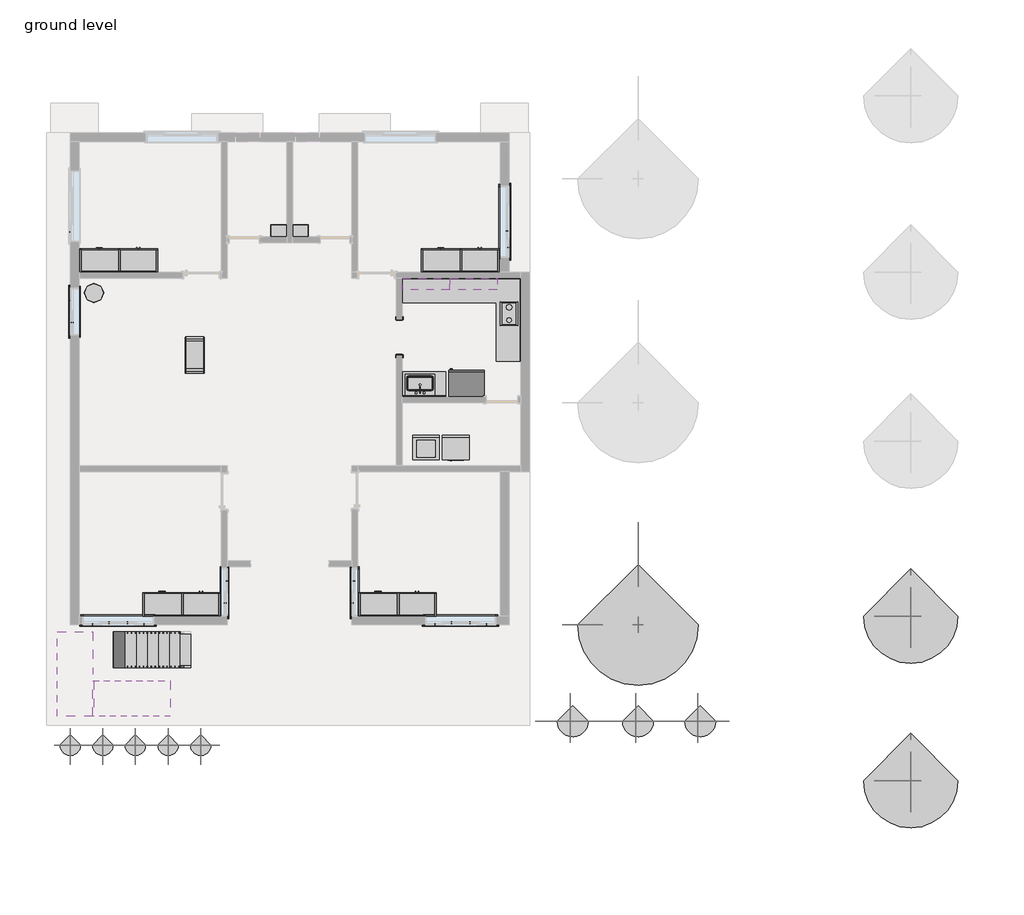
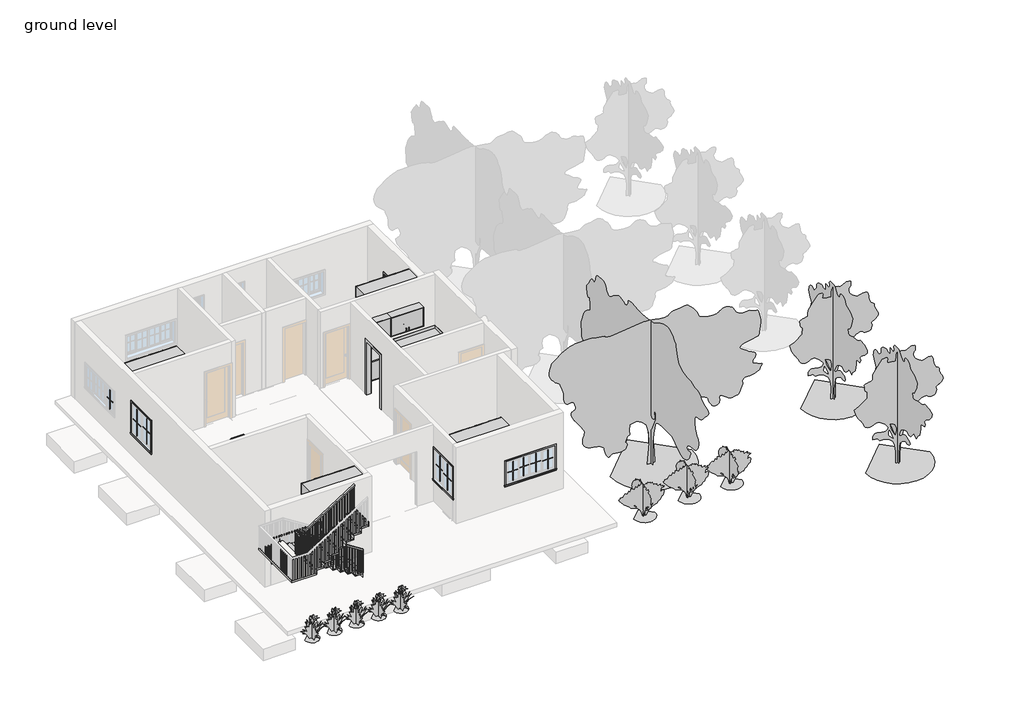
# One storey, part 3 of 4: 33 proxies, 15 furniture elements, 11 geographic elements, 3 flow terminals, 2 stair flights, 1 railing, 1 slab.
"""IFC4 building model written with IfcOpenShell, lengths in millimetres."""

from ifc_helpers import new_model, si_unit, frame, origin, place, context, project, spatial, polyline, outline, extrude, faceted_brep, transform, mapped, element, save
from components import proxy_3c1fa1d0, proxy_97c73763, muntin_pattern_2x2_muntin_pattern_2x2_c2d27229, muntin_pattern_2x2_muntin_pattern_2x2_cf37b409, muntin_pattern_2x2_muntin_pattern_2x2_31a16349, proxy_7dd6dadb, trim_window_exterior_flat_with_sill_ac84ebb5, trim_window_exterior_flat_with_sill_7cfdd449, trim_window_exterior_flat_with_sill_3c945769, trim_window_interior_flat_picture_frame_caf2db4f, trim_window_interior_flat_picture_frame_f1e0b15b, trim_window_interior_flat_picture_frame_0edfbaa2, proxy_e75280ca, flow_terminal_7145266d, flow_terminal_4d548711, furniture_2dca108f, furniture_65fa61b5, furniture_1wardrobe_6271_1wardrobe_6271_4dd35231, furniture_3428e43d, furniture_bf8a676d, furniture_97fe820d, furniture_a6d59748, furniture_f5a42f9b, furniture_9d41381f, furniture_ea954fa4, rpc_plant_tropical_55f6ff97, rpc_plant_tropical_6475341c, rpc_tree_deciduous_common_apple_20_2cf08d23, rpc_tree_deciduous_japanese_cherry_15_e499737d, non_monolithic_landing_d7d9d8c2, stair_flight_7bdf39d0, stair_flight_d241fc77

model = new_model("IFC4")

# Units and contexts
model_context = context("Model", 3, world=origin())
ifc_project = project(units=[si_unit("LENGTHUNIT", "METRE", prefix="MILLI")], contexts=[model_context])

# Site, building, storey
site = spatial("IfcSite", under=ifc_project)
building = spatial("IfcBuilding", under=site)
storey = spatial("IfcBuildingStorey", under=building, Name="ground level", Elevation=609.6)

# Proxies
placement = place(None, origin())
proxy_shape = proxy_3c1fa1d0(model_context)
element("IfcBuildingElementProxy", 1, Name="Cook Top-2 Unit : 12\" x 18\" 2", ObjectType="Cook Top-2 Unit : 12\" x 18\" 2", at=placement, inside=storey, context=model_context, shape_type="MappedRepresentation", body=[
    mapped(proxy_shape, transform((-1440.8124084, 5502.3713848, 609.6), x_axis=(1.0, 0.0, 0.0), y_axis=(0.0, 1.0, 0.0), z_axis=(0.0, 0.0, 1.0))),
])
proxy_2_shape = proxy_97c73763(model_context)
element("IfcBuildingElementProxy", 2, Name="Dryer : 27\" x 25\" x 35\"", ObjectType="Dryer : 27\" x 25\" x 35\"", at=placement, inside=storey, context=model_context, shape_type="MappedRepresentation", body=[
    mapped(proxy_2_shape, transform((-3115.1998647, 1776.2351766, 609.6), x_axis=(1.0, 0.0, 0.0), y_axis=(0.0, 1.0, 0.0), z_axis=(0.0, 0.0, 1.0))),
])
muntin_pattern_2x2_muntin_pattern_2x2_shape = muntin_pattern_2x2_muntin_pattern_2x2_c2d27229(model_context)
element("IfcBuildingElementProxy", 3, Name="Muntin Pattern_2x2 : Muntin Pattern_2x2", ObjectType="Muntin Pattern_2x2 : Muntin Pattern_2x2", at=placement, inside=storey, context=model_context, shape_type="MappedRepresentation", body=[
    mapped(muntin_pattern_2x2_muntin_pattern_2x2_shape, transform((-12588.2374084, 5299.2336804, 1606.55), x_axis=(0.0, -1.0, 0.0), y_axis=(1.0, 0.0, 0.0), z_axis=(0.0, 0.0, 1.0))),
])
element("IfcBuildingElementProxy", 4, Name="Muntin Pattern_2x2 : Muntin Pattern_2x2", ObjectType="Muntin Pattern_2x2 : Muntin Pattern_2x2", at=placement, inside=storey, context=model_context, shape_type="MappedRepresentation", body=[
    mapped(muntin_pattern_2x2_muntin_pattern_2x2_shape, transform((-12632.6874084, 5867.5586804, 1606.55), x_axis=(0.0, -1.0, 0.0), y_axis=(1.0, 0.0, 0.0), z_axis=(0.0, 0.0, 1.0))),
])
muntin_pattern_2x2_muntin_pattern_2x2_2_shape = muntin_pattern_2x2_muntin_pattern_2x2_cf37b409(model_context)
element("IfcBuildingElementProxy", 5, Name="Muntin Pattern_2x2 : Muntin Pattern_2x2", ObjectType="Muntin Pattern_2x2 : Muntin Pattern_2x2", at=placement, inside=storey, context=model_context, shape_type="MappedRepresentation", body=[
    mapped(muntin_pattern_2x2_muntin_pattern_2x2_2_shape, transform((-8657.5874084, -1908.0163196, 1606.55), x_axis=(0.0, -1.0, 0.0), y_axis=(1.0, 0.0, 0.0), z_axis=(0.0, 0.0, 1.0))),
])
element("IfcBuildingElementProxy", 6, Name="Muntin Pattern_2x2 : Muntin Pattern_2x2", ObjectType="Muntin Pattern_2x2 : Muntin Pattern_2x2", at=placement, inside=storey, context=model_context, shape_type="MappedRepresentation", body=[
    mapped(muntin_pattern_2x2_muntin_pattern_2x2_2_shape, transform((-8613.1374084, -1339.6913196, 1606.55), x_axis=(0.0, -1.0, 0.0), y_axis=(1.0, 0.0, 0.0), z_axis=(0.0, 0.0, 1.0))),
])
element("IfcBuildingElementProxy", 7, Name="Muntin Pattern_2x2 : Muntin Pattern_2x2", ObjectType="Muntin Pattern_2x2 : Muntin Pattern_2x2", at=placement, inside=storey, context=model_context, shape_type="MappedRepresentation", body=[
    mapped(muntin_pattern_2x2_muntin_pattern_2x2_2_shape, transform((-5349.2374084, -1339.6913196, 1606.55), x_axis=(0.0, 1.0, 0.0), y_axis=(-1.0, 0.0, 0.0), z_axis=(0.0, 0.0, 1.0))),
])
element("IfcBuildingElementProxy", 8, Name="Muntin Pattern_2x2 : Muntin Pattern_2x2", ObjectType="Muntin Pattern_2x2 : Muntin Pattern_2x2", at=placement, inside=storey, context=model_context, shape_type="MappedRepresentation", body=[
    mapped(muntin_pattern_2x2_muntin_pattern_2x2_2_shape, transform((-5393.6874084, -1908.0163196, 1606.55), x_axis=(0.0, 1.0, 0.0), y_axis=(-1.0, 0.0, 0.0), z_axis=(0.0, 0.0, 1.0))),
])
muntin_pattern_2x2_muntin_pattern_2x2_3_shape = muntin_pattern_2x2_muntin_pattern_2x2_31a16349(model_context)
element("IfcBuildingElementProxy", 9, Name="Muntin Pattern_2x2 : Muntin Pattern_2x2", ObjectType="Muntin Pattern_2x2 : Muntin Pattern_2x2", at=placement, inside=storey, context=model_context, shape_type="MappedRepresentation", body=[
    mapped(muntin_pattern_2x2_muntin_pattern_2x2_3_shape, transform((-12632.6874084, 7634.4461804, 1606.55), x_axis=(0.0, 1.0, 0.0), y_axis=(-1.0, 0.0, 0.0), z_axis=(0.0, 0.0, 1.0))),
])
element("IfcBuildingElementProxy", 10, Name="Muntin Pattern_2x2 : Muntin Pattern_2x2", ObjectType="Muntin Pattern_2x2 : Muntin Pattern_2x2", at=placement, inside=storey, context=model_context, shape_type="MappedRepresentation", body=[
    mapped(muntin_pattern_2x2_muntin_pattern_2x2_3_shape, transform((-1418.5874084, 7659.8461804, 1606.55), x_axis=(0.0, -1.0, 0.0), y_axis=(1.0, 0.0, 0.0), z_axis=(0.0, 0.0, 1.0))),
])
element("IfcBuildingElementProxy", 11, Name="Muntin Pattern_2x2 : Muntin Pattern_2x2", ObjectType="Muntin Pattern_2x2 : Muntin Pattern_2x2", at=placement, inside=storey, context=model_context, shape_type="MappedRepresentation", body=[
    mapped(muntin_pattern_2x2_muntin_pattern_2x2_3_shape, transform((-1374.1374084, 7234.3961804, 1606.55), x_axis=(0.0, -1.0, 0.0), y_axis=(1.0, 0.0, 0.0), z_axis=(0.0, 0.0, 1.0))),
])
element("IfcBuildingElementProxy", 12, Name="Muntin Pattern_2x2 : Muntin Pattern_2x2", ObjectType="Muntin Pattern_2x2 : Muntin Pattern_2x2", at=placement, inside=storey, context=model_context, shape_type="MappedRepresentation", body=[
    mapped(muntin_pattern_2x2_muntin_pattern_2x2_3_shape, transform((-1948.8124084, -2458.8788196, 1606.55), x_axis=(-1.0, 0.0, 0.0), y_axis=(0.0, -1.0, 0.0), z_axis=(0.0, 0.0, 1.0))),
])
element("IfcBuildingElementProxy", 13, Name="Muntin Pattern_2x2 : Muntin Pattern_2x2", ObjectType="Muntin Pattern_2x2 : Muntin Pattern_2x2", at=placement, inside=storey, context=model_context, shape_type="MappedRepresentation", body=[
    mapped(muntin_pattern_2x2_muntin_pattern_2x2_3_shape, transform((-2374.2624084, -2414.4288196, 1606.55), x_axis=(-1.0, 0.0, 0.0), y_axis=(0.0, -1.0, 0.0), z_axis=(0.0, 0.0, 1.0))),
])
element("IfcBuildingElementProxy", 14, Name="Muntin Pattern_2x2 : Muntin Pattern_2x2", ObjectType="Muntin Pattern_2x2 : Muntin Pattern_2x2", at=placement, inside=storey, context=model_context, shape_type="MappedRepresentation", body=[
    mapped(muntin_pattern_2x2_muntin_pattern_2x2_3_shape, transform((-2844.1624084, -2414.4288196, 1606.55), x_axis=(-1.0, 0.0, 0.0), y_axis=(0.0, -1.0, 0.0), z_axis=(0.0, 0.0, 1.0))),
])
element("IfcBuildingElementProxy", 15, Name="Muntin Pattern_2x2 : Muntin Pattern_2x2", ObjectType="Muntin Pattern_2x2 : Muntin Pattern_2x2", at=placement, inside=storey, context=model_context, shape_type="MappedRepresentation", body=[
    mapped(muntin_pattern_2x2_muntin_pattern_2x2_3_shape, transform((-3269.6124084, -2458.8788196, 1606.55), x_axis=(-1.0, 0.0, 0.0), y_axis=(0.0, -1.0, 0.0), z_axis=(0.0, 0.0, 1.0))),
])
element("IfcBuildingElementProxy", 16, Name="Muntin Pattern_2x2 : Muntin Pattern_2x2", ObjectType="Muntin Pattern_2x2 : Muntin Pattern_2x2", at=placement, inside=storey, context=model_context, shape_type="MappedRepresentation", body=[
    mapped(muntin_pattern_2x2_muntin_pattern_2x2_3_shape, transform((-10749.9124084, -2458.8788196, 1606.55), x_axis=(-1.0, 0.0, 0.0), y_axis=(0.0, -1.0, 0.0), z_axis=(0.0, 0.0, 1.0))),
])
element("IfcBuildingElementProxy", 17, Name="Muntin Pattern_2x2 : Muntin Pattern_2x2", ObjectType="Muntin Pattern_2x2 : Muntin Pattern_2x2", at=placement, inside=storey, context=model_context, shape_type="MappedRepresentation", body=[
    mapped(muntin_pattern_2x2_muntin_pattern_2x2_3_shape, transform((-11175.3624084, -2414.4288196, 1606.55), x_axis=(-1.0, 0.0, 0.0), y_axis=(0.0, -1.0, 0.0), z_axis=(0.0, 0.0, 1.0))),
])
element("IfcBuildingElementProxy", 18, Name="Muntin Pattern_2x2 : Muntin Pattern_2x2", ObjectType="Muntin Pattern_2x2 : Muntin Pattern_2x2", at=placement, inside=storey, context=model_context, shape_type="MappedRepresentation", body=[
    mapped(muntin_pattern_2x2_muntin_pattern_2x2_3_shape, transform((-11645.2624084, -2414.4288196, 1606.55), x_axis=(-1.0, 0.0, 0.0), y_axis=(0.0, -1.0, 0.0), z_axis=(0.0, 0.0, 1.0))),
])
element("IfcBuildingElementProxy", 19, Name="Muntin Pattern_2x2 : Muntin Pattern_2x2", ObjectType="Muntin Pattern_2x2 : Muntin Pattern_2x2", at=placement, inside=storey, context=model_context, shape_type="MappedRepresentation", body=[
    mapped(muntin_pattern_2x2_muntin_pattern_2x2_3_shape, transform((-12070.7124084, -2458.8788196, 1606.55), x_axis=(-1.0, 0.0, 0.0), y_axis=(0.0, -1.0, 0.0), z_axis=(0.0, 0.0, 1.0))),
])
proxy_3_shape = proxy_7dd6dadb(model_context)
element("IfcBuildingElementProxy", 20, Name="Passage Opening-Cased : 36\" x 84\"", ObjectType="Passage Opening-Cased : 36\" x 84\"", at=placement, inside=storey, context=model_context, shape_type="MappedRepresentation", body=[
    mapped(proxy_3_shape, transform((-4184.0124084, 4931.1848371, 609.6), x_axis=(0.0, 1.0, 0.0), y_axis=(-1.0, 0.0, 0.0), z_axis=(0.0, 0.0, 1.0))),
])
trim_window_exterior_flat_with_sill_shape = trim_window_exterior_flat_with_sill_ac84ebb5(model_context)
element("IfcBuildingElementProxy", 21, Name="Trim-Window-Exterior-Flat : with Sill", ObjectType="Trim-Window-Exterior-Flat : with Sill", at=placement, inside=storey, context=model_context, shape_type="MappedRepresentation", body=[
    mapped(trim_window_exterior_flat_with_sill_shape, transform((-12642.2124084, 5583.3961804, 2743.2), x_axis=(0.0, 1.0, 0.0), y_axis=(0.0, 0.0, -1.0), z_axis=(-1.0, 0.0, 0.0))),
])
trim_window_exterior_flat_with_sill_2_shape = trim_window_exterior_flat_with_sill_7cfdd449(model_context)
element("IfcBuildingElementProxy", 22, Name="Trim-Window-Exterior-Flat : with Sill", ObjectType="Trim-Window-Exterior-Flat : with Sill", at=placement, inside=storey, context=model_context, shape_type="MappedRepresentation", body=[
    mapped(trim_window_exterior_flat_with_sill_2_shape, transform((-8603.6124084, -1623.8538196, 2743.2), x_axis=(0.0, 1.0, 0.0), y_axis=(0.0, 0.0, 1.0), z_axis=(1.0, 0.0, 0.0))),
])
element("IfcBuildingElementProxy", 23, Name="Trim-Window-Exterior-Flat : with Sill", ObjectType="Trim-Window-Exterior-Flat : with Sill", at=placement, inside=storey, context=model_context, shape_type="MappedRepresentation", body=[
    mapped(trim_window_exterior_flat_with_sill_2_shape, transform((-5403.2124084, -1623.8538196, 2743.2), x_axis=(0.0, -1.0, 0.0), y_axis=(0.0, 0.0, 1.0), z_axis=(-1.0, 0.0, 0.0))),
])
trim_window_exterior_flat_with_sill_3_shape = trim_window_exterior_flat_with_sill_3c945769(model_context)
element("IfcBuildingElementProxy", 24, Name="Trim-Window-Exterior-Flat : with Sill", ObjectType="Trim-Window-Exterior-Flat : with Sill", at=placement, inside=storey, context=model_context, shape_type="MappedRepresentation", body=[
    mapped(trim_window_exterior_flat_with_sill_3_shape, transform((-1364.6124084, 7894.7961804, 2438.4), x_axis=(0.0, 1.0, 0.0), y_axis=(0.0, 0.0, 1.0), z_axis=(1.0, 0.0, 0.0))),
])
element("IfcBuildingElementProxy", 25, Name="Trim-Window-Exterior-Flat : with Sill", ObjectType="Trim-Window-Exterior-Flat : with Sill", at=placement, inside=storey, context=model_context, shape_type="MappedRepresentation", body=[
    mapped(trim_window_exterior_flat_with_sill_3_shape, transform((-2609.2124084, -2468.4038196, 2438.4), x_axis=(1.0, 0.0, 0.0), y_axis=(0.0, 0.0, 1.0), z_axis=(0.0, -1.0, 0.0))),
])
element("IfcBuildingElementProxy", 26, Name="Trim-Window-Exterior-Flat : with Sill", ObjectType="Trim-Window-Exterior-Flat : with Sill", at=placement, inside=storey, context=model_context, shape_type="MappedRepresentation", body=[
    mapped(trim_window_exterior_flat_with_sill_3_shape, transform((-11410.3124084, -2468.4038196, 2438.4), x_axis=(1.0, 0.0, 0.0), y_axis=(0.0, 0.0, 1.0), z_axis=(0.0, -1.0, 0.0))),
])
trim_window_interior_flat_picture_frame_shape = trim_window_interior_flat_picture_frame_caf2db4f(model_context)
element("IfcBuildingElementProxy", 27, Name="Trim-Window-Interior-Flat : Picture Frame", ObjectType="Trim-Window-Interior-Flat : Picture Frame", at=placement, inside=storey, context=model_context, shape_type="MappedRepresentation", body=[
    mapped(trim_window_interior_flat_picture_frame_shape, transform((-12413.6124084, 5583.3961804, 2743.2), x_axis=(0.0, -1.0, 0.0), y_axis=(0.0, 0.0, -1.0), z_axis=(1.0, 0.0, 0.0))),
])
trim_window_interior_flat_picture_frame_2_shape = trim_window_interior_flat_picture_frame_f1e0b15b(model_context)
element("IfcBuildingElementProxy", 28, Name="Trim-Window-Interior-Flat : Picture Frame", ObjectType="Trim-Window-Interior-Flat : Picture Frame", at=placement, inside=storey, context=model_context, shape_type="MappedRepresentation", body=[
    mapped(trim_window_interior_flat_picture_frame_2_shape, transform((-8756.0124084, -1623.8538196, 2743.2), x_axis=(0.0, -1.0, 0.0), y_axis=(0.0, 0.0, 1.0), z_axis=(-1.0, 0.0, 0.0))),
])
element("IfcBuildingElementProxy", 29, Name="Trim-Window-Interior-Flat : Picture Frame", ObjectType="Trim-Window-Interior-Flat : Picture Frame", at=placement, inside=storey, context=model_context, shape_type="MappedRepresentation", body=[
    mapped(trim_window_interior_flat_picture_frame_2_shape, transform((-5250.8124084, -1623.8538196, 2743.2), x_axis=(0.0, 1.0, 0.0), y_axis=(0.0, 0.0, 1.0), z_axis=(1.0, 0.0, 0.0))),
])
trim_window_interior_flat_picture_frame_3_shape = trim_window_interior_flat_picture_frame_0edfbaa2(model_context)
element("IfcBuildingElementProxy", 30, Name="Trim-Window-Interior-Flat : Picture Frame", ObjectType="Trim-Window-Interior-Flat : Picture Frame", at=placement, inside=storey, context=model_context, shape_type="MappedRepresentation", body=[
    mapped(trim_window_interior_flat_picture_frame_3_shape, transform((-1593.2124084, 7894.7961804, 2438.4), x_axis=(0.0, -1.0, 0.0), y_axis=(0.0, 0.0, 1.0), z_axis=(-1.0, 0.0, 0.0))),
])
element("IfcBuildingElementProxy", 31, Name="Trim-Window-Interior-Flat : Picture Frame", ObjectType="Trim-Window-Interior-Flat : Picture Frame", at=placement, inside=storey, context=model_context, shape_type="MappedRepresentation", body=[
    mapped(trim_window_interior_flat_picture_frame_3_shape, transform((-2609.2124084, -2239.8038196, 2438.4), x_axis=(-1.0, 0.0, 0.0), y_axis=(0.0, 0.0, 1.0), z_axis=(0.0, 1.0, 0.0))),
])
element("IfcBuildingElementProxy", 32, Name="Trim-Window-Interior-Flat : Picture Frame", ObjectType="Trim-Window-Interior-Flat : Picture Frame", at=placement, inside=storey, context=model_context, shape_type="MappedRepresentation", body=[
    mapped(trim_window_interior_flat_picture_frame_3_shape, transform((-11410.3124084, -2239.8038196, 2438.4), x_axis=(-1.0, 0.0, 0.0), y_axis=(0.0, 0.0, 1.0), z_axis=(0.0, 1.0, 0.0))),
])
proxy_4_shape = proxy_e75280ca(model_context)
element("IfcBuildingElementProxy", 33, Name="Washer : 27\" x 25\" x 35\"", ObjectType="Washer : 27\" x 25\" x 35\"", at=placement, inside=storey, context=model_context, shape_type="MappedRepresentation", body=[
    mapped(proxy_4_shape, transform((-3918.6298768, 1811.7466156, 609.6), x_axis=(1.0, 0.0, 0.0), y_axis=(0.0, 1.0, 0.0), z_axis=(0.0, 0.0, 1.0))),
])

# Flow terminals
flow_terminal_shape = flow_terminal_7145266d(model_context)
element("IfcFlowTerminal", 34, ObjectType="Sink - Work : 20\"x18\" 2", at=placement, inside=storey, context=model_context, shape_type="MappedRepresentation", body=[
    mapped(flow_terminal_shape, transform((-7282.8124084, 7513.7961804, 1524.0), x_axis=(-1.0, 0.0, 0.0), y_axis=(0.0, -1.0, 0.0), z_axis=(0.0, 0.0, 1.0))),
])
element("IfcFlowTerminal", 35, ObjectType="Sink - Work : 20\"x18\" 2", at=placement, inside=storey, context=model_context, shape_type="MappedRepresentation", body=[
    mapped(flow_terminal_shape, transform((-6724.0124084, 7513.7961804, 1524.0), x_axis=(-1.0, 0.0, 0.0), y_axis=(0.0, -1.0, 0.0), z_axis=(0.0, 0.0, 1.0))),
])
flow_terminal_2_shape = flow_terminal_4d548711(model_context)
element("IfcFlowTerminal", 36, ObjectType="Sink Kitchen-Single : 30\" x 21\"", at=placement, inside=storey, context=model_context, shape_type="MappedRepresentation", body=[
    mapped(flow_terminal_2_shape, transform((-3634.9231678, 3706.1415815, 609.6), x_axis=(-1.0, 0.0, 0.0), y_axis=(0.0, -1.0, 0.0), z_axis=(0.0, 0.0, 1.0))),
])

# Furniture
furniture_shape = furniture_2dca108f(model_context)
element("IfcFurniture", 37, at=placement, inside=storey, context=model_context, shape_type="MappedRepresentation", body=[
    mapped(furniture_shape, transform((-9441.8124084, 4465.7961804, 609.6), x_axis=(1.0, 0.0, 0.0), y_axis=(0.0, 1.0, 0.0), z_axis=(0.0, 0.0, 1.0))),
])
furniture_2_shape = furniture_65fa61b5(model_context)
element("IfcFurniture", 38, at=placement, inside=storey, context=model_context, shape_type="MappedRepresentation", body=[
    mapped(furniture_2_shape, transform((-3066.4124084, 3411.6961804, 609.6), x_axis=(-1.0, 0.0, 0.0), y_axis=(0.0, -1.0, 0.0), z_axis=(0.0, 0.0, 1.0))),
])
furniture_1wardrobe_6271_1wardrobe_6271_shape = furniture_1wardrobe_6271_1wardrobe_6271_4dd35231(model_context)
element("IfcFurniture", 39, ObjectType="1Wardrobe_6271 : 1Wardrobe_6271", at=placement, inside=storey, context=model_context, shape_type="MappedRepresentation", body=[
    mapped(furniture_1wardrobe_6271_1wardrobe_6271_shape, transform((-10394.3124084, 6599.3961804, 609.6), x_axis=(-1.0, 0.0, 0.0), y_axis=(0.0, -1.0, 0.0), z_axis=(0.0, 0.0, 1.0))),
])
element("IfcFurniture", 40, ObjectType="1Wardrobe_6271 : 1Wardrobe_6271", at=placement, inside=storey, context=model_context, shape_type="MappedRepresentation", body=[
    mapped(furniture_1wardrobe_6271_1wardrobe_6271_shape, transform((-1618.6124084, 6599.3961804, 609.6), x_axis=(-1.0, 0.0, 0.0), y_axis=(0.0, -1.0, 0.0), z_axis=(0.0, 0.0, 1.0))),
])
element("IfcFurniture", 41, ObjectType="1Wardrobe_6271 : 1Wardrobe_6271", at=placement, inside=storey, context=model_context, shape_type="MappedRepresentation", body=[
    mapped(furniture_1wardrobe_6271_1wardrobe_6271_shape, transform((-3231.5124084, -2239.8038196, 609.6), x_axis=(-1.0, 0.0, 0.0), y_axis=(0.0, -1.0, 0.0), z_axis=(0.0, 0.0, 1.0))),
])
element("IfcFurniture", 42, ObjectType="1Wardrobe_6271 : 1Wardrobe_6271", at=placement, inside=storey, context=model_context, shape_type="MappedRepresentation", body=[
    mapped(furniture_1wardrobe_6271_1wardrobe_6271_shape, transform((-8781.4124084, -2239.8038196, 609.6), x_axis=(-1.0, 0.0, 0.0), y_axis=(0.0, -1.0, 0.0), z_axis=(0.0, 0.0, 1.0))),
])
furniture_3_shape = furniture_3428e43d(model_context)
element("IfcFurniture", 43, ObjectType="48\" 2", at=placement, inside=storey, context=model_context, shape_type="MappedRepresentation", body=[
    mapped(furniture_3_shape, transform((-2674.6573683, 6446.9961804, 609.6), x_axis=(1.0, 0.0, 0.0), y_axis=(0.0, 1.0, 0.0), z_axis=(0.0, 0.0, 1.0))),
])
element("IfcFurniture", 44, ObjectType="48\" 3", at=placement, inside=storey, context=model_context, shape_type="MappedRepresentation", body=[
    mapped(furniture_3_shape, transform((-1059.8124084, 5013.8411403, 609.6), x_axis=(0.0, -1.0, 0.0), y_axis=(1.0, 0.0, 0.0), z_axis=(0.0, 0.0, 1.0))),
])
furniture_4_shape = furniture_bf8a676d(model_context)
element("IfcFurniture", 45, ObjectType="Base Cabinet-Combo01 : 30\" 2", at=placement, inside=storey, context=model_context, shape_type="MappedRepresentation", body=[
    mapped(furniture_4_shape, transform((-3669.3501133, 6446.9961804, 609.6), x_axis=(1.0, 0.0, 0.0), y_axis=(0.0, 1.0, 0.0), z_axis=(0.0, 0.0, 1.0))),
])
furniture_5_shape = furniture_97fe820d(model_context)
element("IfcFurniture", 46, ObjectType="Base Cabinet-Corner Unit-Square : 36\"", at=placement, inside=storey, context=model_context, shape_type="MappedRepresentation", body=[
    mapped(furniture_5_shape, transform((-1586.5501133, 6446.9961804, 609.6), x_axis=(1.0, 0.0, 0.0), y_axis=(0.0, 1.0, 0.0), z_axis=(0.0, 0.0, 1.0))),
])
furniture_6_shape = furniture_a6d59748(model_context)
element("IfcFurniture", 47, ObjectType="Counter Top w Sink Hole : 24\" Depth", at=placement, inside=storey, context=model_context, shape_type="MappedRepresentation", body=[
    mapped(furniture_6_shape, transform((-4190.6747034, 3398.9961804, 609.6), x_axis=(-1.0, 0.0, 0.0), y_axis=(0.0, -1.0, 0.0), z_axis=(0.0, 0.0, 1.0))),
])
furniture_7_shape = furniture_f5a42f9b(model_context)
element("IfcFurniture", 48, ObjectType="Counter Top-L Shaped : 24\" Depth", at=placement, inside=storey, context=model_context, shape_type="MappedRepresentation", body=[
    mapped(furniture_7_shape, transform((-1059.8124084, 5246.5338853, 609.6), x_axis=(0.0, -1.0, 0.0), y_axis=(1.0, 0.0, 0.0), z_axis=(0.0, 0.0, 1.0))),
])
furniture_8_shape = furniture_9d41381f(model_context)
element("IfcFurniture", 49, ObjectType="Table-Trio End : 20\" Diameter", at=placement, inside=storey, context=model_context, shape_type="MappedRepresentation", body=[
    mapped(furniture_8_shape, transform((-12032.6124084, 6065.9961804, 609.6), x_axis=(1.0, 0.0, 0.0), y_axis=(0.0, 1.0, 0.0), z_axis=(0.0, 0.0, 1.0))),
])
furniture_9_shape = furniture_ea954fa4(model_context)
element("IfcFurniture", 50, ObjectType="Upper Cabinet-Pass-Thru : 48\" x 30\" x 12\"", at=placement, inside=storey, context=model_context, shape_type="MappedRepresentation", body=[
    mapped(furniture_9_shape, transform((-3516.9501133, 6446.9961804, 609.6), x_axis=(1.0, 0.0, 0.0), y_axis=(0.0, 1.0, 0.0), z_axis=(0.0, 0.0, 1.0))),
])
element("IfcFurniture", 51, ObjectType="Upper Cabinet-Pass-Thru : 48\" x 30\" x 12\"", at=placement, inside=storey, context=model_context, shape_type="MappedRepresentation", body=[
    mapped(furniture_9_shape, transform((-2297.7501133, 6446.9961804, 609.6), x_axis=(1.0, 0.0, 0.0), y_axis=(0.0, 1.0, 0.0), z_axis=(0.0, 0.0, 1.0))),
])

# Geographic elements
rpc_plant_tropical_shape = rpc_plant_tropical_55f6ff97(model_context)
element("IfcGeographicElement", 52, ObjectType="RPC Plant - Tropical", at=placement, inside=storey, context=model_context, shape_type="MappedRepresentation", body=[
    mapped(rpc_plant_tropical_shape, transform((-12642.2124084, -5554.5038196, 457.2), x_axis=(1.0, 0.0, 0.0), y_axis=(0.0, 1.0, 0.0), z_axis=(0.0, 0.0, 1.0))),
])
element("IfcGeographicElement", 53, ObjectType="RPC Plant - Tropical", at=placement, inside=storey, context=model_context, shape_type="MappedRepresentation", body=[
    mapped(rpc_plant_tropical_shape, transform((-11804.0124084, -5554.5038196, 457.2), x_axis=(1.0, 0.0, 0.0), y_axis=(0.0, 1.0, 0.0), z_axis=(0.0, 0.0, 1.0))),
])
element("IfcGeographicElement", 54, ObjectType="RPC Plant - Tropical", at=placement, inside=storey, context=model_context, shape_type="MappedRepresentation", body=[
    mapped(rpc_plant_tropical_shape, transform((-10127.6124084, -5554.5038196, 457.2), x_axis=(1.0, 0.0, 0.0), y_axis=(0.0, 1.0, 0.0), z_axis=(0.0, 0.0, 1.0))),
])
element("IfcGeographicElement", 55, ObjectType="RPC Plant - Tropical", at=placement, inside=storey, context=model_context, shape_type="MappedRepresentation", body=[
    mapped(rpc_plant_tropical_shape, transform((-9289.4124084, -5554.5038196, 457.2), x_axis=(1.0, 0.0, 0.0), y_axis=(0.0, 1.0, 0.0), z_axis=(0.0, 0.0, 1.0))),
])
element("IfcGeographicElement", 56, ObjectType="RPC Plant - Tropical", at=placement, inside=storey, context=model_context, shape_type="MappedRepresentation", body=[
    mapped(rpc_plant_tropical_shape, transform((-10965.8124084, -5554.5038196, 457.2), x_axis=(1.0, 0.0, 0.0), y_axis=(0.0, 1.0, 0.0), z_axis=(0.0, 0.0, 1.0))),
])
rpc_plant_tropical_2_shape = rpc_plant_tropical_6475341c(model_context)
element("IfcGeographicElement", 57, ObjectType="RPC Plant - Tropical", at=placement, inside=storey, context=model_context, shape_type="MappedRepresentation", body=[
    mapped(rpc_plant_tropical_2_shape, transform((273.6875916, -4944.9038196, 457.2), x_axis=(1.0, 0.0, 0.0), y_axis=(0.0, 1.0, 0.0), z_axis=(0.0, 0.0, 1.0))),
])
element("IfcGeographicElement", 58, ObjectType="RPC Plant - Tropical", at=placement, inside=storey, context=model_context, shape_type="MappedRepresentation", body=[
    mapped(rpc_plant_tropical_2_shape, transform((3550.2875916, -4944.9038196, 609.6), x_axis=(1.0, 0.0, 0.0), y_axis=(0.0, 1.0, 0.0), z_axis=(0.0, 0.0, 1.0))),
])
element("IfcGeographicElement", 59, ObjectType="RPC Plant - Tropical", at=placement, inside=storey, context=model_context, shape_type="MappedRepresentation", body=[
    mapped(rpc_plant_tropical_2_shape, transform((1950.0875916, -4944.9038196, 609.6), x_axis=(1.0, 0.0, 0.0), y_axis=(0.0, 1.0, 0.0), z_axis=(0.0, 0.0, 1.0))),
])
rpc_tree_deciduous_common_apple_20_shape = rpc_tree_deciduous_common_apple_20_2cf08d23(model_context)
element("IfcGeographicElement", 60, ObjectType="RPC Tree - Deciduous : Common Apple - 20'", at=placement, inside=storey, context=model_context, shape_type="MappedRepresentation", body=[
    mapped(rpc_tree_deciduous_common_apple_20_shape, transform((1950.0875916, -2468.4038196, 457.2), x_axis=(1.0, 0.0, 0.0), y_axis=(0.0, 1.0, 0.0), z_axis=(0.0, 0.0, 1.0))),
])
rpc_tree_deciduous_japanese_cherry_15_shape = rpc_tree_deciduous_japanese_cherry_15_e499737d(model_context)
element("IfcGeographicElement", 61, ObjectType="RPC Tree - Deciduous : Japanese Cherry - 15'", at=placement, inside=storey, context=model_context, shape_type="MappedRepresentation", body=[
    mapped(rpc_tree_deciduous_japanese_cherry_15_shape, transform((8960.4875916, -2239.8038196, 457.2), x_axis=(1.0, 0.0, 0.0), y_axis=(0.0, 1.0, 0.0), z_axis=(0.0, 0.0, 1.0))),
])
element("IfcGeographicElement", 62, ObjectType="RPC Tree - Deciduous : Japanese Cherry - 15'", at=placement, inside=storey, context=model_context, shape_type="MappedRepresentation", body=[
    mapped(rpc_tree_deciduous_japanese_cherry_15_shape, transform((8960.4875916, -6468.9038196, 457.2), x_axis=(1.0, 0.0, 0.0), y_axis=(0.0, 1.0, 0.0), z_axis=(0.0, 0.0, 1.0))),
])

# Railing
element("IfcRailing", 63, ObjectType="Handrail - Rectangular", at=placement, inside=storey, context=model_context, shape_type="SolidModel", body=[
    faceted_brep([(-9543.8120641, -3562.3669819, 1701.8), (-9543.8120641, -3562.3669819, 1641.586276), (-9543.8120641, -3511.5669819, 1641.586276), (-9543.8120641, -3511.5669819, 1701.8), (-11982.2120641, -3562.3669819, 3253.5090909), (-12033.0120641, -3562.3669819, 3225.6226396), (-12033.0120641, -3511.5669819, 3225.6226396), (-11982.2120641, -3511.5669819, 3253.5090909), (-11982.2120641, -3562.3669819, 3302.0), (-12033.0120641, -3562.3669819, 3251.2), (-12033.0120641, -3511.5669819, 3251.2), (-11982.2120641, -3511.5669819, 3302.0), (-12058.4120641, -3562.3669819, 3302.0), (-12058.4120641, -3562.3669819, 3251.2), (-12109.2120641, -3511.5669819, 3251.2), (-12109.2120641, -3511.5669819, 3302.0), (-12058.4120641, -3638.5669819, 3302.0), (-12058.4120641, -3638.5669819, 3251.2), (-12109.2120641, -3638.5669819, 3251.2), (-12109.2120641, -3638.5669819, 3302.0), (-12058.4120641, -3827.3038196, 3302.0), (-12058.4120641, -3878.1038196, 3251.2), (-12109.2120641, -3878.1038196, 3251.2), (-12109.2120641, -3827.3038196, 3302.0), (-12058.4120641, -3827.3038196, 3528.2909091), (-12058.4120641, -3878.1038196, 3477.4909091), (-12109.2120641, -3878.1038196, 3477.4909091), (-12109.2120641, -3827.3038196, 3528.2909091), (-12058.4120641, -3903.5038196, 3528.2909091), (-12058.4120641, -3903.5038196, 3477.4909091), (-12109.2120641, -3954.3038196, 3477.4909091), (-12109.2120641, -3954.3038196, 3528.2909091), (-11982.2120641, -3903.5038196, 3528.2909091), (-11967.4190691, -3903.5038196, 3477.4909091), (-11967.4190691, -3954.3038196, 3477.4909091), (-11982.2120641, -3954.3038196, 3528.2909091), (-10102.6120641, -3903.5038196, 4724.4), (-10102.6120641, -3954.3038196, 4724.4), (-10102.6120641, -3954.3038196, 4664.186276), (-10102.6120641, -3903.5038196, 4664.186276)], [[[0, 1, 2, 3]], [[1, 0, 4, 5]], [[2, 1, 5, 6]], [[3, 2, 6, 7]], [[0, 3, 7, 4]], [[5, 4, 8, 9]], [[6, 5, 9, 10]], [[7, 6, 10, 11]], [[4, 7, 11, 8]], [[9, 8, 12, 13]], [[10, 9, 13, 14]], [[11, 10, 14, 15]], [[8, 11, 15, 12]], [[13, 12, 16, 17]], [[14, 13, 17, 18]], [[15, 14, 18, 19]], [[12, 15, 19, 16]], [[17, 16, 20, 21]], [[18, 17, 21, 22]], [[19, 18, 22, 23]], [[16, 19, 23, 20]], [[21, 20, 24, 25]], [[22, 21, 25, 26]], [[23, 22, 26, 27]], [[20, 23, 27, 24]], [[25, 24, 28, 29]], [[26, 25, 29, 30]], [[27, 26, 30, 31]], [[24, 27, 31, 28]], [[29, 28, 32, 33]], [[30, 29, 33, 34]], [[31, 30, 34, 35]], [[28, 31, 35, 32]], [[36, 37, 38, 39]], [[33, 32, 36, 39]], [[34, 33, 39, 38]], [[35, 34, 38, 37]], [[32, 35, 37, 36]]]),
    extrude(outline(polyline([(4625.7976396, -10162.9370641), (3632.2, -10162.9370641), (3632.2, -10143.8870641), (4637.9203669, -10143.8870641), (4625.7976396, -10162.9370641)])), frame((0.0, -3938.4288196, 0.0), z_axis=(0.0, 1.0, 0.0), x_axis=(0.0, 0.0, 1.0)), (0.0, 0.0, 1.0), 19.05),
    extrude(outline(polyline([(4561.1430941, -10264.5370641), (3632.2, -10264.5370641), (3632.2, -10245.4870641), (4573.2658214, -10245.4870641), (4561.1430941, -10264.5370641)])), frame((0.0, -3938.4288196, 0.0), z_axis=(0.0, 1.0, 0.0), x_axis=(0.0, 0.0, 1.0)), (0.0, 0.0, 1.0), 19.05),
    extrude(outline(polyline([(4496.4885487, -10366.1370641), (3632.2, -10366.1370641), (3632.2, -10347.0870641), (4508.611276, -10347.0870641), (4496.4885487, -10366.1370641)])), frame((0.0, -3938.4288196, 0.0), z_axis=(0.0, 1.0, 0.0), x_axis=(0.0, 0.0, 1.0)), (0.0, 0.0, 1.0), 19.05),
    extrude(outline(polyline([(4431.8340032, -10467.7370641), (3454.4, -10467.7370641), (3454.4, -10448.6870641), (4443.9567305, -10448.6870641), (4431.8340032, -10467.7370641)])), frame((0.0, -3938.4288196, 0.0), z_axis=(0.0, 1.0, 0.0), x_axis=(0.0, 0.0, 1.0)), (0.0, 0.0, 1.0), 19.05),
    extrude(outline(polyline([(4367.1794578, -10569.3370641), (3454.4, -10569.3370641), (3454.4, -10550.2870641), (4379.3021851, -10550.2870641), (4367.1794578, -10569.3370641)])), frame((0.0, -3938.4288196, 0.0), z_axis=(0.0, 1.0, 0.0), x_axis=(0.0, 0.0, 1.0)), (0.0, 0.0, 1.0), 19.05),
    extrude(outline(polyline([(4302.5249123, -10670.9370641), (3454.4, -10670.9370641), (3454.4, -10651.8870641), (4314.6476396, -10651.8870641), (4302.5249123, -10670.9370641)])), frame((0.0, -3938.4288196, 0.0), z_axis=(0.0, 1.0, 0.0), x_axis=(0.0, 0.0, 1.0)), (0.0, 0.0, 1.0), 19.05),
    extrude(outline(polyline([(4237.8703669, -10772.5370641), (3276.6, -10772.5370641), (3276.6, -10753.4870641), (4249.9930941, -10753.4870641), (4237.8703669, -10772.5370641)])), frame((0.0, -3938.4288196, 0.0), z_axis=(0.0, 1.0, 0.0), x_axis=(0.0, 0.0, 1.0)), (0.0, 0.0, 1.0), 19.05),
    extrude(outline(polyline([(4173.2158214, -10874.1370641), (3276.6, -10874.1370641), (3276.6, -10855.0870641), (4185.3385487, -10855.0870641), (4173.2158214, -10874.1370641)])), frame((0.0, -3938.4288196, 0.0), z_axis=(0.0, 1.0, 0.0), x_axis=(0.0, 0.0, 1.0)), (0.0, 0.0, 1.0), 19.05),
    extrude(outline(polyline([(4108.561276, -10975.7370641), (3098.8, -10975.7370641), (3098.8, -10956.6870641), (4120.6840032, -10956.6870641), (4108.561276, -10975.7370641)])), frame((0.0, -3938.4288196, 0.0), z_axis=(0.0, 1.0, 0.0), x_axis=(0.0, 0.0, 1.0)), (0.0, 0.0, 1.0), 19.05),
    extrude(outline(polyline([(4043.9067305, -11077.3370641), (3098.8, -11077.3370641), (3098.8, -11058.2870641), (4056.0294578, -11058.2870641), (4043.9067305, -11077.3370641)])), frame((0.0, -3938.4288196, 0.0), z_axis=(0.0, 1.0, 0.0), x_axis=(0.0, 0.0, 1.0)), (0.0, 0.0, 1.0), 19.05),
    extrude(outline(polyline([(3979.2521851, -11178.9370641), (3098.8, -11178.9370641), (3098.8, -11159.8870641), (3991.3749123, -11159.8870641), (3979.2521851, -11178.9370641)])), frame((0.0, -3938.4288196, 0.0), z_axis=(0.0, 1.0, 0.0), x_axis=(0.0, 0.0, 1.0)), (0.0, 0.0, 1.0), 19.05),
    extrude(outline(polyline([(3914.5976396, -11280.5370641), (2921.0, -11280.5370641), (2921.0, -11261.4870641), (3926.7203669, -11261.4870641), (3914.5976396, -11280.5370641)])), frame((0.0, -3938.4288196, 0.0), z_axis=(0.0, 1.0, 0.0), x_axis=(0.0, 0.0, 1.0)), (0.0, 0.0, 1.0), 19.05),
    extrude(outline(polyline([(3849.9430941, -11382.1370641), (2921.0, -11382.1370641), (2921.0, -11363.0870641), (3862.0658214, -11363.0870641), (3849.9430941, -11382.1370641)])), frame((0.0, -3938.4288196, 0.0), z_axis=(0.0, 1.0, 0.0), x_axis=(0.0, 0.0, 1.0)), (0.0, 0.0, 1.0), 19.05),
    extrude(outline(polyline([(3785.2885487, -11483.7370641), (2921.0, -11483.7370641), (2921.0, -11464.6870641), (3797.411276, -11464.6870641), (3785.2885487, -11483.7370641)])), frame((0.0, -3938.4288196, 0.0), z_axis=(0.0, 1.0, 0.0), x_axis=(0.0, 0.0, 1.0)), (0.0, 0.0, 1.0), 19.05),
    extrude(outline(polyline([(3720.6340032, -11585.3370641), (2743.2, -11585.3370641), (2743.2, -11566.2870641), (3732.7567305, -11566.2870641), (3720.6340032, -11585.3370641)])), frame((0.0, -3938.4288196, 0.0), z_axis=(0.0, 1.0, 0.0), x_axis=(0.0, 0.0, 1.0)), (0.0, 0.0, 1.0), 19.05),
    extrude(outline(polyline([(3655.9794578, -11686.9370641), (2743.2, -11686.9370641), (2743.2, -11667.8870641), (3668.1021851, -11667.8870641), (3655.9794578, -11686.9370641)])), frame((0.0, -3938.4288196, 0.0), z_axis=(0.0, 1.0, 0.0), x_axis=(0.0, 0.0, 1.0)), (0.0, 0.0, 1.0), 19.05),
    extrude(outline(polyline([(3591.3249123, -11788.5370641), (2743.2, -11788.5370641), (2743.2, -11769.4870641), (3603.4476396, -11769.4870641), (3591.3249123, -11788.5370641)])), frame((0.0, -3938.4288196, 0.0), z_axis=(0.0, 1.0, 0.0), x_axis=(0.0, 0.0, 1.0)), (0.0, 0.0, 1.0), 19.05),
    extrude(outline(polyline([(3526.6703669, -11890.1370641), (2565.4, -11890.1370641), (2565.4, -11871.0870641), (3538.7930941, -11871.0870641), (3526.6703669, -11890.1370641)])), frame((0.0, -3938.4288196, 0.0), z_axis=(0.0, 1.0, 0.0), x_axis=(0.0, 0.0, 1.0)), (0.0, 0.0, 1.0), 19.05),
    extrude(outline(polyline([(3462.0158214, -11991.7370641), (2565.4, -11991.7370641), (2565.4, -11972.6870641), (3474.1385487, -11972.6870641), (3462.0158214, -11991.7370641)])), frame((0.0, -3938.4288196, 0.0), z_axis=(0.0, 1.0, 0.0), x_axis=(0.0, 0.0, 1.0)), (0.0, 0.0, 1.0), 19.05),
    extrude(outline(polyline([(-12074.2870641, -3832.2419819), (-12074.2870641, -3851.2919819), (-12093.3370641, -3851.2919819), (-12093.3370641, -3832.2419819), (-12074.2870641, -3832.2419819)])), frame((0.0, 0.0, 2387.6), z_axis=(0.0, 0.0, 1.0), x_axis=(1.0, 0.0, 0.0)), (0.0, 0.0, 1.0), 1089.8909091),
    extrude(outline(polyline([(-12074.2870641, -3730.6419819), (-12074.2870641, -3749.6919819), (-12093.3370641, -3749.6919819), (-12093.3370641, -3730.6419819), (-12074.2870641, -3730.6419819)])), frame((0.0, 0.0, 2387.6), z_axis=(0.0, 0.0, 1.0), x_axis=(1.0, 0.0, 0.0)), (0.0, 0.0, 1.0), 863.6),
    extrude(outline(polyline([(-12074.2870641, -3629.0419819), (-12074.2870641, -3648.0919819), (-12093.3370641, -3648.0919819), (-12093.3370641, -3629.0419819), (-12074.2870641, -3629.0419819)])), frame((0.0, 0.0, 2387.6), z_axis=(0.0, 0.0, 1.0), x_axis=(1.0, 0.0, 0.0)), (0.0, 0.0, 1.0), 863.6),
    extrude(outline(polyline([(3199.3567305, -11991.7370641), (2209.8, -11991.7370641), (2209.8, -11972.6870641), (3187.2340032, -11972.6870641), (3199.3567305, -11991.7370641)])), frame((0.0, -3546.4919819, 0.0), z_axis=(0.0, 1.0, 0.0), x_axis=(0.0, 0.0, 1.0)), (0.0, 0.0, 1.0), 19.05),
    extrude(outline(polyline([(3134.7021851, -11890.1370641), (2209.8, -11890.1370641), (2209.8, -11871.0870641), (3122.5794578, -11871.0870641), (3134.7021851, -11890.1370641)])), frame((0.0, -3546.4919819, 0.0), z_axis=(0.0, 1.0, 0.0), x_axis=(0.0, 0.0, 1.0)), (0.0, 0.0, 1.0), 19.05),
    extrude(outline(polyline([(3070.0476396, -11788.5370641), (2209.8, -11788.5370641), (2209.8, -11769.4870641), (3057.9249123, -11769.4870641), (3070.0476396, -11788.5370641)])), frame((0.0, -3546.4919819, 0.0), z_axis=(0.0, 1.0, 0.0), x_axis=(0.0, 0.0, 1.0)), (0.0, 0.0, 1.0), 19.05),
    extrude(outline(polyline([(3005.3930941, -11686.9370641), (2032.0, -11686.9370641), (2032.0, -11667.8870641), (2993.2703669, -11667.8870641), (3005.3930941, -11686.9370641)])), frame((0.0, -3546.4919819, 0.0), z_axis=(0.0, 1.0, 0.0), x_axis=(0.0, 0.0, 1.0)), (0.0, 0.0, 1.0), 19.05),
    extrude(outline(polyline([(2940.7385487, -11585.3370641), (2032.0, -11585.3370641), (2032.0, -11566.2870641), (2928.6158214, -11566.2870641), (2940.7385487, -11585.3370641)])), frame((0.0, -3546.4919819, 0.0), z_axis=(0.0, 1.0, 0.0), x_axis=(0.0, 0.0, 1.0)), (0.0, 0.0, 1.0), 19.05),
    extrude(outline(polyline([(2876.0840032, -11483.7370641), (1854.2, -11483.7370641), (1854.2, -11464.6870641), (2863.961276, -11464.6870641), (2876.0840032, -11483.7370641)])), frame((0.0, -3546.4919819, 0.0), z_axis=(0.0, 1.0, 0.0), x_axis=(0.0, 0.0, 1.0)), (0.0, 0.0, 1.0), 19.05),
    extrude(outline(polyline([(2811.4294578, -11382.1370641), (1854.2, -11382.1370641), (1854.2, -11363.0870641), (2799.3067305, -11363.0870641), (2811.4294578, -11382.1370641)])), frame((0.0, -3546.4919819, 0.0), z_axis=(0.0, 1.0, 0.0), x_axis=(0.0, 0.0, 1.0)), (0.0, 0.0, 1.0), 19.05),
    extrude(outline(polyline([(2746.7749123, -11280.5370641), (1854.2, -11280.5370641), (1854.2, -11261.4870641), (2734.6521851, -11261.4870641), (2746.7749123, -11280.5370641)])), frame((0.0, -3546.4919819, 0.0), z_axis=(0.0, 1.0, 0.0), x_axis=(0.0, 0.0, 1.0)), (0.0, 0.0, 1.0), 19.05),
    extrude(outline(polyline([(2682.1203669, -11178.9370641), (1676.4, -11178.9370641), (1676.4, -11159.8870641), (2669.9976396, -11159.8870641), (2682.1203669, -11178.9370641)])), frame((0.0, -3546.4919819, 0.0), z_axis=(0.0, 1.0, 0.0), x_axis=(0.0, 0.0, 1.0)), (0.0, 0.0, 1.0), 19.05),
    extrude(outline(polyline([(2617.4658214, -11077.3370641), (1676.4, -11077.3370641), (1676.4, -11058.2870641), (2605.3430941, -11058.2870641), (2617.4658214, -11077.3370641)])), frame((0.0, -3546.4919819, 0.0), z_axis=(0.0, 1.0, 0.0), x_axis=(0.0, 0.0, 1.0)), (0.0, 0.0, 1.0), 19.05),
    extrude(outline(polyline([(2552.811276, -10975.7370641), (1676.4, -10975.7370641), (1676.4, -10956.6870641), (2540.6885487, -10956.6870641), (2552.811276, -10975.7370641)])), frame((0.0, -3546.4919819, 0.0), z_axis=(0.0, 1.0, 0.0), x_axis=(0.0, 0.0, 1.0)), (0.0, 0.0, 1.0), 19.05),
    extrude(outline(polyline([(2488.1567305, -10874.1370641), (1498.6, -10874.1370641), (1498.6, -10855.0870641), (2476.0340032, -10855.0870641), (2488.1567305, -10874.1370641)])), frame((0.0, -3546.4919819, 0.0), z_axis=(0.0, 1.0, 0.0), x_axis=(0.0, 0.0, 1.0)), (0.0, 0.0, 1.0), 19.05),
    extrude(outline(polyline([(2423.5021851, -10772.5370641), (1498.6, -10772.5370641), (1498.6, -10753.4870641), (2411.3794578, -10753.4870641), (2423.5021851, -10772.5370641)])), frame((0.0, -3546.4919819, 0.0), z_axis=(0.0, 1.0, 0.0), x_axis=(0.0, 0.0, 1.0)), (0.0, 0.0, 1.0), 19.05),
    extrude(outline(polyline([(2358.8476396, -10670.9370641), (1498.6, -10670.9370641), (1498.6, -10651.8870641), (2346.7249123, -10651.8870641), (2358.8476396, -10670.9370641)])), frame((0.0, -3546.4919819, 0.0), z_axis=(0.0, 1.0, 0.0), x_axis=(0.0, 0.0, 1.0)), (0.0, 0.0, 1.0), 19.05),
    extrude(outline(polyline([(2294.1930941, -10569.3370641), (1320.8, -10569.3370641), (1320.8, -10550.2870641), (2282.0703669, -10550.2870641), (2294.1930941, -10569.3370641)])), frame((0.0, -3546.4919819, 0.0), z_axis=(0.0, 1.0, 0.0), x_axis=(0.0, 0.0, 1.0)), (0.0, 0.0, 1.0), 19.05),
    extrude(outline(polyline([(2229.5385487, -10467.7370641), (1320.8, -10467.7370641), (1320.8, -10448.6870641), (2217.4158214, -10448.6870641), (2229.5385487, -10467.7370641)])), frame((0.0, -3546.4919819, 0.0), z_axis=(0.0, 1.0, 0.0), x_axis=(0.0, 0.0, 1.0)), (0.0, 0.0, 1.0), 19.05),
    extrude(outline(polyline([(2164.8840032, -10366.1370641), (1143.0, -10366.1370641), (1143.0, -10347.0870641), (2152.761276, -10347.0870641), (2164.8840032, -10366.1370641)])), frame((0.0, -3546.4919819, 0.0), z_axis=(0.0, 1.0, 0.0), x_axis=(0.0, 0.0, 1.0)), (0.0, 0.0, 1.0), 19.05),
    extrude(outline(polyline([(2100.2294578, -10264.5370641), (1143.0, -10264.5370641), (1143.0, -10245.4870641), (2088.1067305, -10245.4870641), (2100.2294578, -10264.5370641)])), frame((0.0, -3546.4919819, 0.0), z_axis=(0.0, 1.0, 0.0), x_axis=(0.0, 0.0, 1.0)), (0.0, 0.0, 1.0), 19.05),
    extrude(outline(polyline([(2035.5749123, -10162.9370641), (1143.0, -10162.9370641), (1143.0, -10143.8870641), (2023.4521851, -10143.8870641), (2035.5749123, -10162.9370641)])), frame((0.0, -3546.4919819, 0.0), z_axis=(0.0, 1.0, 0.0), x_axis=(0.0, 0.0, 1.0)), (0.0, 0.0, 1.0), 19.05),
    extrude(outline(polyline([(1970.9203669, -10061.3370641), (965.2, -10061.3370641), (965.2, -10042.2870641), (1958.7976396, -10042.2870641), (1970.9203669, -10061.3370641)])), frame((0.0, -3546.4919819, 0.0), z_axis=(0.0, 1.0, 0.0), x_axis=(0.0, 0.0, 1.0)), (0.0, 0.0, 1.0), 19.05),
    extrude(outline(polyline([(1906.2658214, -9959.7370641), (965.2, -9959.7370641), (965.2, -9940.6870641), (1894.1430941, -9940.6870641), (1906.2658214, -9959.7370641)])), frame((0.0, -3546.4919819, 0.0), z_axis=(0.0, 1.0, 0.0), x_axis=(0.0, 0.0, 1.0)), (0.0, 0.0, 1.0), 19.05),
    extrude(outline(polyline([(1841.611276, -9858.1370641), (965.2, -9858.1370641), (965.2, -9839.0870641), (1829.4885487, -9839.0870641), (1841.611276, -9858.1370641)])), frame((0.0, -3546.4919819, 0.0), z_axis=(0.0, 1.0, 0.0), x_axis=(0.0, 0.0, 1.0)), (0.0, 0.0, 1.0), 19.05),
    extrude(outline(polyline([(1776.9567305, -9756.5370641), (787.4, -9756.5370641), (787.4, -9737.4870641), (1764.8340032, -9737.4870641), (1776.9567305, -9756.5370641)])), frame((0.0, -3546.4919819, 0.0), z_axis=(0.0, 1.0, 0.0), x_axis=(0.0, 0.0, 1.0)), (0.0, 0.0, 1.0), 19.05),
    extrude(outline(polyline([(1712.3021851, -9654.9370641), (787.4, -9654.9370641), (787.4, -9635.8870641), (1700.1794578, -9635.8870641), (1712.3021851, -9654.9370641)])), frame((0.0, -3546.4919819, 0.0), z_axis=(0.0, 1.0, 0.0), x_axis=(0.0, 0.0, 1.0)), (0.0, 0.0, 1.0), 19.05),
    extrude(outline(polyline([(-12074.2870641, -3919.3788196), (-12074.2870641, -3938.4288196), (-12093.3370641, -3938.4288196), (-12093.3370641, -3919.3788196), (-12074.2870641, -3919.3788196)])), frame((0.0, 0.0, 2387.6), z_axis=(0.0, 0.0, 1.0), x_axis=(1.0, 0.0, 0.0)), (0.0, 0.0, 1.0), 1089.8909091),
    extrude(outline(polyline([(-12074.2870641, -3546.4919819), (-12093.3370641, -3546.4919819), (-12093.3370641, -3527.4419819), (-12074.2870641, -3527.4419819), (-12074.2870641, -3546.4919819)])), frame((0.0, 0.0, 2387.6), z_axis=(0.0, 0.0, 1.0), x_axis=(1.0, 0.0, 0.0)), (0.0, 0.0, 1.0), 863.6),
    extrude(outline(polyline([(4652.0635487, -10121.6620641), (3632.2, -10121.6620641), (3632.2, -10102.6120641), (4664.186276, -10102.6120641), (4652.0635487, -10121.6620641)])), frame((0.0, -3938.4288196, 0.0), z_axis=(0.0, 1.0, 0.0), x_axis=(0.0, 0.0, 1.0)), (0.0, 0.0, 1.0), 19.05),
    extrude(outline(polyline([(1653.7090032, -9562.8620641), (787.4, -9562.8620641), (787.4, -9543.8120641), (1641.586276, -9543.8120641), (1653.7090032, -9562.8620641)])), frame((0.0, -3546.4919819, 0.0), z_axis=(0.0, 1.0, 0.0), x_axis=(0.0, 0.0, 1.0)), (0.0, 0.0, 1.0), 19.05),
])

# Slab
non_monolithic_landing_shape = non_monolithic_landing_d7d9d8c2(model_context)
element("IfcSlab", 64, ObjectType="Non-Monolithic Landing", at=placement, inside=storey, context=model_context, shape_type="MappedRepresentation", body=[
    mapped(non_monolithic_landing_shape, transform((0.0, 0.0, 0.0), x_axis=(1.0, 0.0, 0.0), y_axis=(0.0, 1.0, 0.0), z_axis=(0.0, 0.0, 1.0))),
])

# Stair flights
stair_flight_shape = stair_flight_7bdf39d0(model_context)
element("IfcStairFlight", 65, ObjectType="2\" Tread 1\" Nosing 1/4\" Riser", at=placement, inside=storey, context=model_context, shape_type="MappedRepresentation", body=[
    mapped(stair_flight_shape, transform((0.0, 0.0, 0.0), x_axis=(1.0, 0.0, 0.0), y_axis=(0.0, 1.0, 0.0), z_axis=(0.0, 0.0, 1.0))),
])
stair_flight_2_shape = stair_flight_d241fc77(model_context)
element("IfcStairFlight", 66, ObjectType="2\" Tread 1\" Nosing 1/4\" Riser", at=placement, inside=storey, context=model_context, shape_type="MappedRepresentation", body=[
    mapped(stair_flight_2_shape, transform((0.0, 0.0, 0.0), x_axis=(1.0, 0.0, 0.0), y_axis=(0.0, 1.0, 0.0), z_axis=(0.0, 0.0, 1.0))),
])

save(model, "model.ifc")

# Revit data of these elements
# Type "Cook Top-2 Unit : 12\" x 18\" 2"
#   Assembly Code = "E1090400"
#   Counter Height = 3' - 0"
#   Depth = 2' - 0"
#   Width = 1' - 6"
#   Burner Material = Metal - Chrome
#   Cooktop Material = Metal - Steel, Polished
#   Default Elevation = 0
# Type "Dryer : 27\" x 25\" x 35\""
#   Label = "D"
#   Assembly Code = "E1090400"
#   Depth = 2' - 1"
#   Height = 2' - 11"
#   Width = 2' - 3"
#   Dryer Material = Metal - Paint Finish - Ivory,Glossy
#   Default Elevation = 0
# Type "Muntin Pattern_2x2 : Muntin Pattern_2x2"
#   Width [instance default] = 4' - 0"
#   Thickness = 0' - 0 1/2"
#   Height [instance default] = 4' - 0"
#   Distance = 0' - 0 3/4"
#   Interior Material [instance default] = none
#   Exterior Material [instance default] = none
#   Default Elevation = 0
# Type "Passage Opening-Cased : 36\" x 84\""
#   Height = 7' - 0"
#   Trim Thickness = 0' - 0 3/4"
#   Trim Width = 0' - 3"
#   Width = 3' - 0"
#   Frame Material = Door - Frame
#   Default Elevation = 0
# Type "Trim-Window-Exterior-Flat : with Sill"
#   Trim Width = 0' - 2 1/4"
#   Trim Thickness_Picture Frame = 0' - 1 1/4"
#   Trim Thickness_with Sill = 0' - 0 3/4"
#   Sill Thickness = 0' - 1 1/4"
#   Opening Width [instance default] = 2' - 0"
#   Opening Height [instance default] = 3' - 0"
#   Default Elevation = 4' - 0"
#   Sill = yes
#   Picture Frame = no
#   Trim Material [instance default] = none
# Type "Trim-Window-Interior-Flat : Picture Frame"
#   Trim Thickness_Picture Frame = 0' - 1 1/4"
#   Trim Width = 0' - 2 1/4"
#   Trim Thickness_with Sill = 0' - 0 3/4"
#   Sill Thickness = 0' - 1 1/4"
#   Opening Width [instance default] = 2' - 0"
#   Opening Height [instance default] = 3' - 0"
#   Default Elevation = 4' - 0"
#   Sill = no
#   Picture Frame = yes
#   Trim Material [instance default] = none
# Type "Washer : 27\" x 25\" x 35\""
#   Label = "W"
#   Assembly Code = "E1090400"
#   Depth = 2' - 1"
#   Height = 2' - 11"
#   Width = 2' - 3"
#   Washer Material = Metal - Paint Finish - Ivory,Matte
#   Default Elevation = 0
# Type "Sink - Work : 20\"x18\" 2"
#   WFU = 2
#   Sink Width = 1' - 0"
#   Sink Length = 1' - 4"
#   Sink Depth = 0' - 8"
#   Sanitary Radius = 3/4"
#   Sanitary Diameter = 1 1/2"
#   Hot Water Radius = 1/4"
#   Hot Water Diameter = 1/2"
#   HWFU = 2.25
#   Flow Pressure [instance default] = 8.00 psi
#   Faucet Height = 1' - 1 5/8"
#   Cold Water Radius = 1/4"
#   Cold Water Diameter = 1/2"
#   CWFU = 2.25
#   Sink Material = none
#   Faucet Material = none
#   Default Elevation = 0
# Type "Sink Kitchen-Single : 30\" x 21\""
#   Assembly Code = "D2010410"
#   Counter Height = 3' - 0"
#   Depth = 1' - 9"
#   Width = 2' - 6"
#   Faucet Material = Steel, Polished
#   Sink Material = Steel, Polished
#   Default Elevation = 0
# Type
#   Default Elevation = 0
# Type
#   Default Elevation = 0
# Type "1Wardrobe_6271 : 1Wardrobe_6271"
#   Default Elevation = 0
# Type "48\" 2"
#   Assembly Code = "C1030410"
#   Depth = 2' - 0"
#   Height = 2' - 10 1/2"
#   Toe Depth = 0' - 3"
#   Toe Height = 0' - 3 1/2"
#   Width = 4' - 0"
#   Cabinet Material = none
#   Door/Drawer Material = none
#   Handle Material = Cabinets - Handles
#   Default Elevation = 0
# Type "48\" 3"
#   Assembly Code = "C1030410"
#   Depth = 2' - 0"
#   Height = 2' - 10 1/2"
#   Toe Depth = 0' - 3"
#   Toe Height = 0' - 3 1/2"
#   Width = 4' - 0"
#   Cabinet Material = none
#   Door/Drawer Material = none
#   Handle Material = Cabinets - Handles
#   Default Elevation = 0
# Type "Base Cabinet-Combo01 : 30\" 2"
#   Depth = 1' - 10"
#   Height = 2' - 10 1/2"
#   Toe Depth = 0' - 3"
#   Toe Height = 0' - 3 1/2"
#   Width = 3' - 0"
#   Default Elevation = 0
# Type "Base Cabinet-Corner Unit-Square : 36\""
#   Assembly Code = "C1030410"
#   Depth = 2' - 0"
#   Height = 2' - 10 1/2"
#   Toe Depth = 0' - 3"
#   Toe Height = 0' - 3 1/2"
#   Width = 3' - 0"
#   Cabinet Material = Cabinets
#   Door/Drawer Material = Cabinets
#   Handle Material = Cabinets - Handles
#   Default Elevation = 0
# Type "Counter Top w Sink Hole : 24\" Depth"
#   Assembly Code = "C1030400"
#   Counter Thickness = 0' - 1 1/2"
#   Depth = 2' - 1"
#   Height = 3' - 0"
#   Length [instance default] = 8' - 0"
#   Sink Location [instance default] = 2' - 0"
#   Sink Location To Wall [instance default] = 0' - 6"
#   Sink Opening Depth [instance default] = 1' - 3"
#   Sink Opening Width [instance default] = 2' - 3"
#   Counter Top Material = none
#   Default Elevation = 0
# Type "Counter Top-L Shaped : 24\" Depth"
#   Assembly Code = "C1030400"
#   Counter Thickness = 0' - 1 1/2"
#   Depth = 2' - 1"
#   Height = 3' - 0"
#   Length - Leg 1 [instance default] = 8' - 0"
#   Length - Leg 2 [instance default] = 6' - 0"
#   Counter Top Material = none
#   Default Elevation = 0
# Type "Table-Trio End : 20\" Diameter"
#   Assembly Code = "E2020200"
#   Base and Trim Material = Wood - Birch
#   Table Top Material = Laminate - Ivory,Matte
#   Default Elevation = 0
# Type "Upper Cabinet-Pass-Thru : 48\" x 30\" x 12\""
#   Depth = 1' - 0"
#   Height = 2' - 6"
#   Top of Cabinet = 7' - 0"
#   Width = 4' - 0"
#   Default Elevation = 0
# Type "RPC Plant - Tropical"
